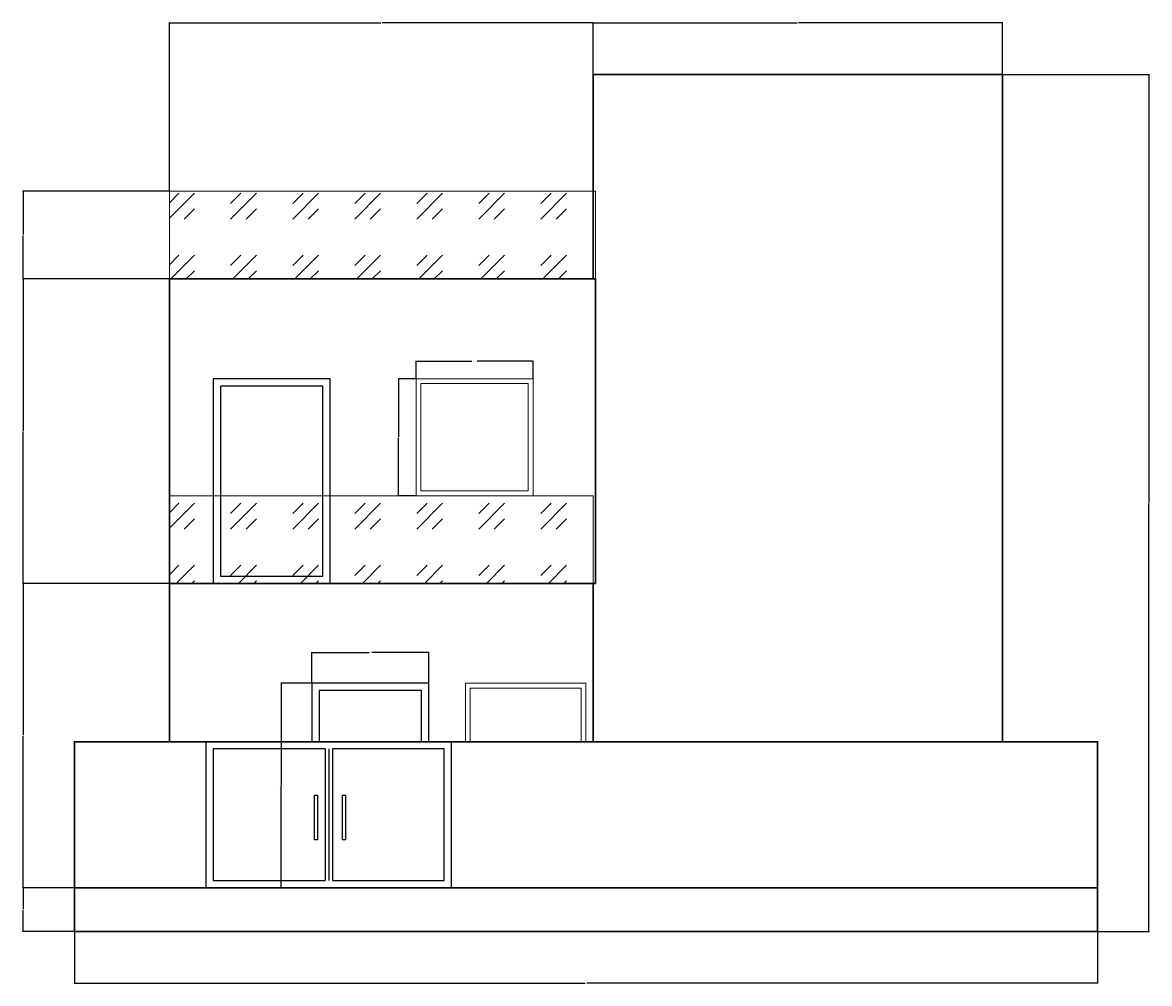
# Model space of a CAD drawing. Units: inches. Extents: x 810 to 2232, y 728 to 1827.
# Tile 4 of 6: x 1317 to 1780, y 1201 to 1596. Entities that reach past the tile are written whole.
import ezdxf

# ---------------------------------------------------------------- set-up
doc = ezdxf.new("R2010")
doc.units = ezdxf.units.IN
for name, color, linetype, lineweight in [('A-ANNO-DIMS', 2, 'Continuous', 18), ('A-ELEV', 7, 'Continuous', 30), ('A-ELEV-DOOR', 7, 'Continuous', 25), ('A-ELEV-GATE', 7, 'Continuous', 25), ('A-ELEV-GLAZ', 7, 'Continuous', 18), ('A-ELEV-PATT', 8, 'Continuous', 13), ('A-ELEV-SITE', 7, 'Continuous', 30)]:
    doc.layers.add(name, color=color, linetype=linetype, lineweight=lineweight)
doc.styles.get("Standard").update_dxf_attribs({"font": 'arial.ttf'})
doc.dimstyles.get("Standard").update_dxf_attribs({"dimtxt": 0.18, "dimasz": 0.18, "dimexe": 0.18, "dimexo": 0.0625, "dimgap": 0.09, "dimtad": 0, "dimtih": 1, "dimtoh": 1, "dimdec": 4, "dimzin": 0, "dimdsep": 46, "dimtxsty": 'Standard', "dimcen": 0.09, "dimadec": 0, "dimazin": 0, "dimtfac": 1, "dimtdec": 4, "dimtofl": 0, "dimtmove": 0, "dimatfit": 3, "dimfxl": 1, "dimtolj": 1, "dimtzin": 0, "dimarcsym": 0})
pattern_1 = [(45, (-481.11, 598.717), (25.45584, 0), [15, -21]), (45, (-474.746, 598.717), (25.45584, 0), [6, -30]), (45, (-481.11, 605.081), (25.45584, 0), [6, -30])]

# ---------------------------------------------------------------- blocks, each defined once
blk = doc.blocks.new('GATE-DOUBLE-ELEV')
for p, q in [((48.89, 57), (48.89, 3)), ((50.39, 57), (50.39, 3)), ((51.89, 57), (51.89, 3))]:
    blk.add_line(p, q)
for points in [[(0, 0), (100.77, 0), (100.77, 60), (0, 60)], [(44.48, 38.04), (45.81, 38.04), (45.81, 19.7), (44.48, 19.7)], [(55.99, 38.04), (57.32, 38.04), (57.32, 19.7), (55.99, 19.7)]]:
    blk.add_lwpolyline(points, close=True)
for points in [[(48.89, 57), (3, 57), (3, 3), (48.89, 3)], [(51.89, 3), (97.77, 3), (97.77, 57), (51.89, 57)]]:
    blk.add_lwpolyline(points)
blk = doc.blocks.new('DOOR-ENTRY-ELEV-SCREENED')
for points in [[(48, 60), (48, 84), (0, 84), (0, 60)], [(45, 60), (45, 81), (3, 81), (3, 60)], [(0, 0), (48, 0)]]:
    blk.add_lwpolyline(points)
blk = doc.blocks.new('WIN-ELEV-SCREENED')
for points in [[(0, 0), (0, 24), (49.5, 24), (49.5, 0)], [(2, 0), (2, 22), (47.5, 22), (47.5, 0)]]:
    blk.add_lwpolyline(points)
blk = doc.blocks.new('DOOR-BALCONY-ELEV')
for points in [[(0, 0), (48, 0), (48, 84), (0, 84)], [(3, 3), (45, 3), (45, 81), (3, 81)]]:
    blk.add_lwpolyline(points, close=True)
blk = doc.blocks.new('WIN-ELEV-SQUARE')
for points in [[(0, 0), (48, 0), (48, 48), (0, 48)], [(2, 2), (46, 2), (46, 46), (2, 46)]]:
    blk.add_lwpolyline(points, close=True)
blk = doc.blocks.new('*D43')
at = {"layer": 'A-ANNO-DIMS', "color": 0, "lineweight": -2, "transparency": 16777216}
for p, q in [((1435.94, 1324.56), (1423.23, 1324.56)), ((1423.41, 1324.38), (1423.41, 1282.74)), ((1423.41, 1240.74), (1423.41, 1282.37)), ((1435.94, 1240.56), (1423.23, 1240.56))]:
    blk.add_line(p, q, dxfattribs=at)
at = {"layer": 'A-ANNO-DIMS', "color": 0, "transparency": 16777216}
for points in [[(1423.38, 1324.38), (1423.44, 1324.38), (1423.41, 1324.56)], [(1423.38, 1240.74), (1423.44, 1240.74), (1423.41, 1240.56)]]:
    blk.add_solid(points, dxfattribs=at)
at = {"layer": 'Defpoints', "color": 0, "transparency": 16777216}
for p in [(1423.41, 1324.56), (1436.01, 1324.56), (1436.01, 1240.56)]:
    blk.add_point(p, dxfattribs=at)
at = {"layer": 'A-ANNO-DIMS', "color": 0, "transparency": 16777216, "insert": (1423.41, 1282.56), "char_height": 0.18, "attachment_point": 5}
blk.add_mtext('\\A1;ENTRY DOOR 84 TYP.', dxfattribs=at)
blk = doc.blocks.new('*D44')
at = {"layer": 'A-ANNO-DIMS', "color": 0, "lineweight": -2, "transparency": 16777216}
for p, q in [((1436.01, 1324.62), (1436.01, 1337.34)), ((1436.19, 1337.16), (1459.48, 1337.16)), ((1483.83, 1337.16), (1460.54, 1337.16)), ((1484.01, 1324.62), (1484.01, 1337.34))]:
    blk.add_line(p, q, dxfattribs=at)
at = {"layer": 'A-ANNO-DIMS', "color": 0, "transparency": 16777216}
for points in [[(1436.19, 1337.19), (1436.19, 1337.13), (1436.01, 1337.16)], [(1483.83, 1337.19), (1483.83, 1337.13), (1484.01, 1337.16)]]:
    blk.add_solid(points, dxfattribs=at)
at = {"layer": 'Defpoints', "color": 0, "transparency": 16777216}
for p in [(1484.01, 1337.16), (1436.01, 1324.56), (1484.01, 1324.56)]:
    blk.add_point(p, dxfattribs=at)
at = {"layer": 'A-ANNO-DIMS', "color": 0, "transparency": 16777216, "insert": (1460.01, 1337.16), "char_height": 0.18, "attachment_point": 5}
blk.add_mtext('\\A1;48 TYP.', dxfattribs=at)
blk = doc.blocks.new('*D49')
at = {"layer": 'A-ANNO-DIMS', "color": 0, "lineweight": -2, "transparency": 16777216}
for p, q in [((1478.76, 1449.62), (1478.76, 1456.94)), ((1478.94, 1456.76), (1501.64, 1456.76)), ((1526.58, 1456.76), (1503.88, 1456.76)), ((1526.76, 1449.62), (1526.76, 1456.94))]:
    blk.add_line(p, q, dxfattribs=at)
at = {"layer": 'A-ANNO-DIMS', "color": 0, "transparency": 16777216}
for points in [[(1478.94, 1456.79), (1478.94, 1456.73), (1478.76, 1456.76)], [(1526.58, 1456.79), (1526.58, 1456.73), (1526.76, 1456.76)]]:
    blk.add_solid(points, dxfattribs=at)
at = {"layer": 'Defpoints', "color": 0, "transparency": 16777216}
for p in [(1526.76, 1456.76), (1478.76, 1449.56), (1526.76, 1449.56)]:
    blk.add_point(p, dxfattribs=at)
at = {"layer": 'A-ANNO-DIMS', "color": 0, "transparency": 16777216, "insert": (1502.76, 1456.76), "char_height": 0.18, "attachment_point": 5}
blk.add_mtext('\\A1;WINDOW 48 TYP.', dxfattribs=at)
blk = doc.blocks.new('*D50')
at = {"layer": 'A-ANNO-DIMS', "color": 0, "lineweight": -2, "transparency": 16777216}
for p, q in [((1478.69, 1449.56), (1471.38, 1449.56)), ((1471.56, 1449.38), (1471.56, 1425.74)), ((1471.56, 1401.74), (1471.56, 1425.38)), ((1478.69, 1401.56), (1471.38, 1401.56))]:
    blk.add_line(p, q, dxfattribs=at)
at = {"layer": 'A-ANNO-DIMS', "color": 0, "transparency": 16777216}
for points in [[(1471.53, 1449.38), (1471.59, 1449.38), (1471.56, 1449.56)], [(1471.53, 1401.74), (1471.59, 1401.74), (1471.56, 1401.56)]]:
    blk.add_solid(points, dxfattribs=at)
at = {"layer": 'Defpoints', "color": 0, "transparency": 16777216}
for p in [(1471.56, 1449.56), (1478.76, 1449.56), (1478.76, 1401.56)]:
    blk.add_point(p, dxfattribs=at)
at = {"layer": 'A-ANNO-DIMS', "color": 0, "transparency": 16777216, "insert": (1471.56, 1425.56), "char_height": 0.18, "attachment_point": 5}
blk.add_mtext('\\A1;48 TYP.', dxfattribs=at)
blk = doc.blocks.new('*D75')
at = {"layer": 'A-ANNO-DIMS', "color": 0, "lineweight": -2, "transparency": 16777216}
for p, q in [((1338.51, 1222.5), (1338.51, 1201.28)), ((1758.51, 1222.5), (1758.51, 1201.28)), ((1338.69, 1201.46), (1548.21, 1201.46)), ((1758.33, 1201.46), (1548.8, 1201.46))]:
    blk.add_line(p, q, dxfattribs=at)
at = {"layer": 'A-ANNO-DIMS', "color": 0, "transparency": 16777216}
for points in [[(1338.69, 1201.49), (1338.69, 1201.43), (1338.51, 1201.46)], [(1758.33, 1201.49), (1758.33, 1201.43), (1758.51, 1201.46)]]:
    blk.add_solid(points, dxfattribs=at)
at = {"layer": 'Defpoints', "color": 0, "transparency": 16777216}
for p in [(1338.51, 1222.56), (1758.51, 1222.56), (1758.51, 1201.46)]:
    blk.add_point(p, dxfattribs=at)
at = {"layer": 'A-ANNO-DIMS', "color": 0, "transparency": 16777216, "insert": (1548.51, 1201.46), "char_height": 0.18, "attachment_point": 5}
blk.add_mtext('\\A1;420', dxfattribs=at)
blk = doc.blocks.new('*D76')
at = {"layer": 'A-ANNO-DIMS', "color": 0, "lineweight": -2, "transparency": 16777216}
for p, q in [((1719.57, 1574.56), (1779.79, 1574.56)), ((1779.61, 1574.38), (1779.61, 1398.74)), ((1779.61, 1222.74), (1779.61, 1398.38)), ((1758.57, 1222.56), (1779.79, 1222.56))]:
    blk.add_line(p, q, dxfattribs=at)
at = {"layer": 'A-ANNO-DIMS', "color": 0, "transparency": 16777216}
for points in [[(1779.58, 1574.38), (1779.64, 1574.38), (1779.61, 1574.56)], [(1779.58, 1222.74), (1779.64, 1222.74), (1779.61, 1222.56)]]:
    blk.add_solid(points, dxfattribs=at)
at = {"layer": 'Defpoints', "color": 0, "transparency": 16777216}
for p in [(1719.51, 1574.56), (1779.61, 1574.56), (1758.51, 1222.56)]:
    blk.add_point(p, dxfattribs=at)
at = {"layer": 'A-ANNO-DIMS', "color": 0, "transparency": 16777216, "insert": (1779.61, 1398.56), "char_height": 0.18, "attachment_point": 5}
blk.add_mtext('\\A1;352', dxfattribs=at)
blk = doc.blocks.new('*D77')
at = {"layer": 'A-ANNO-DIMS', "color": 0, "lineweight": -2, "transparency": 16777216}
for p, q in [((1338.44, 1240.56), (1317.23, 1240.56)), ((1317.41, 1240.38), (1317.41, 1231.74)), ((1317.41, 1222.74), (1317.41, 1231.38)), ((1338.44, 1222.56), (1317.23, 1222.56))]:
    blk.add_line(p, q, dxfattribs=at)
at = {"layer": 'A-ANNO-DIMS', "color": 0, "transparency": 16777216}
for points in [[(1317.38, 1240.38), (1317.44, 1240.38), (1317.41, 1240.56)], [(1317.38, 1222.74), (1317.44, 1222.74), (1317.41, 1222.56)]]:
    blk.add_solid(points, dxfattribs=at)
at = {"layer": 'Defpoints', "color": 0, "transparency": 16777216}
for p in [(1317.41, 1240.56), (1338.51, 1240.56), (1338.51, 1222.56)]:
    blk.add_point(p, dxfattribs=at)
at = {"layer": 'A-ANNO-DIMS', "color": 0, "transparency": 16777216, "insert": (1317.41, 1231.56), "char_height": 0.18, "attachment_point": 5}
blk.add_mtext('\\A1;18', dxfattribs=at)
blk = doc.blocks.new('*D78')
at = {"layer": 'A-ANNO-DIMS', "color": 0, "lineweight": -2, "transparency": 16777216}
for p, q in [((1377.44, 1365.56), (1317.23, 1365.56)), ((1317.41, 1365.38), (1317.41, 1303.24)), ((1317.41, 1240.74), (1317.41, 1302.88)), ((1338.44, 1240.56), (1317.23, 1240.56))]:
    blk.add_line(p, q, dxfattribs=at)
at = {"layer": 'A-ANNO-DIMS', "color": 0, "transparency": 16777216}
for points in [[(1317.38, 1365.38), (1317.44, 1365.38), (1317.41, 1365.56)], [(1317.38, 1240.74), (1317.44, 1240.74), (1317.41, 1240.56)]]:
    blk.add_solid(points, dxfattribs=at)
at = {"layer": 'Defpoints', "color": 0, "transparency": 16777216}
for p in [(1317.41, 1365.56), (1377.51, 1365.56), (1338.51, 1240.56)]:
    blk.add_point(p, dxfattribs=at)
at = {"layer": 'A-ANNO-DIMS', "color": 0, "transparency": 16777216, "insert": (1317.41, 1303.06), "char_height": 0.18, "attachment_point": 5}
blk.add_mtext('\\A1;125', dxfattribs=at)
blk = doc.blocks.new('*D79')
at = {"layer": 'A-ANNO-DIMS', "color": 0, "lineweight": -2, "transparency": 16777216}
for p, q in [((1377.44, 1490.56), (1317.23, 1490.56)), ((1317.41, 1490.38), (1317.41, 1428.24)), ((1317.41, 1365.74), (1317.41, 1427.88)), ((1377.44, 1365.56), (1317.23, 1365.56))]:
    blk.add_line(p, q, dxfattribs=at)
at = {"layer": 'A-ANNO-DIMS', "color": 0, "transparency": 16777216}
for points in [[(1317.38, 1490.38), (1317.44, 1490.38), (1317.41, 1490.56)], [(1317.38, 1365.74), (1317.44, 1365.74), (1317.41, 1365.56)]]:
    blk.add_solid(points, dxfattribs=at)
at = {"layer": 'Defpoints', "color": 0, "transparency": 16777216}
for p in [(1317.41, 1490.56), (1377.51, 1490.56), (1377.51, 1365.56)]:
    blk.add_point(p, dxfattribs=at)
at = {"layer": 'A-ANNO-DIMS', "color": 0, "transparency": 16777216, "insert": (1317.41, 1428.06), "char_height": 0.18, "attachment_point": 5}
blk.add_mtext('\\A1;125', dxfattribs=at)
blk = doc.blocks.new('*D80')
at = {"layer": 'A-ANNO-DIMS', "color": 0, "lineweight": -2, "transparency": 16777216}
for p, q in [((1377.44, 1526.56), (1317.23, 1526.56)), ((1317.41, 1526.38), (1317.41, 1508.74)), ((1317.41, 1490.74), (1317.41, 1508.38)), ((1377.44, 1490.56), (1317.23, 1490.56))]:
    blk.add_line(p, q, dxfattribs=at)
at = {"layer": 'A-ANNO-DIMS', "color": 0, "transparency": 16777216}
for points in [[(1317.38, 1526.38), (1317.44, 1526.38), (1317.41, 1526.56)], [(1317.38, 1490.74), (1317.44, 1490.74), (1317.41, 1490.56)]]:
    blk.add_solid(points, dxfattribs=at)
at = {"layer": 'Defpoints', "color": 0, "transparency": 16777216}
for p in [(1317.41, 1526.56), (1377.51, 1526.56), (1377.51, 1490.56)]:
    blk.add_point(p, dxfattribs=at)
at = {"layer": 'A-ANNO-DIMS', "color": 0, "transparency": 16777216, "insert": (1317.41, 1508.56), "char_height": 0.18, "attachment_point": 5}
blk.add_mtext('\\A1;36', dxfattribs=at)
blk = doc.blocks.new('*D81')
at = {"layer": 'A-ANNO-DIMS', "color": 0, "lineweight": -2, "transparency": 16777216}
for p, q in [((1377.51, 1526.62), (1377.51, 1595.84)), ((1377.69, 1595.66), (1464.23, 1595.66)), ((1551.33, 1595.66), (1464.79, 1595.66)), ((1551.51, 1574.62), (1551.51, 1595.84))]:
    blk.add_line(p, q, dxfattribs=at)
at = {"layer": 'A-ANNO-DIMS', "color": 0, "transparency": 16777216}
for points in [[(1377.69, 1595.69), (1377.69, 1595.63), (1377.51, 1595.66)], [(1551.33, 1595.69), (1551.33, 1595.63), (1551.51, 1595.66)]]:
    blk.add_solid(points, dxfattribs=at)
at = {"layer": 'Defpoints', "color": 0, "transparency": 16777216}
for p in [(1551.51, 1595.66), (1551.51, 1574.56), (1377.51, 1526.56)]:
    blk.add_point(p, dxfattribs=at)
at = {"layer": 'A-ANNO-DIMS', "color": 0, "transparency": 16777216, "insert": (1464.51, 1595.66), "char_height": 0.18, "attachment_point": 5}
blk.add_mtext('\\A1;174', dxfattribs=at)
blk = doc.blocks.new('*D82')
at = {"layer": 'A-ANNO-DIMS', "color": 0, "lineweight": -2, "transparency": 16777216}
for p, q in [((1551.51, 1574.62), (1551.51, 1595.84)), ((1551.69, 1595.66), (1635.23, 1595.66)), ((1719.33, 1595.66), (1635.79, 1595.66)), ((1719.51, 1574.62), (1719.51, 1595.84))]:
    blk.add_line(p, q, dxfattribs=at)
at = {"layer": 'A-ANNO-DIMS', "color": 0, "transparency": 16777216}
for points in [[(1551.69, 1595.69), (1551.69, 1595.63), (1551.51, 1595.66)], [(1719.33, 1595.69), (1719.33, 1595.63), (1719.51, 1595.66)]]:
    blk.add_solid(points, dxfattribs=at)
at = {"layer": 'Defpoints', "color": 0, "transparency": 16777216}
for p in [(1719.51, 1595.66), (1551.51, 1574.56), (1719.51, 1574.56)]:
    blk.add_point(p, dxfattribs=at)
at = {"layer": 'A-ANNO-DIMS', "color": 0, "transparency": 16777216, "insert": (1635.51, 1595.66), "char_height": 0.18, "attachment_point": 5}
blk.add_mtext('\\A1;168', dxfattribs=at)

msp = doc.modelspace()

# ---------------------------------------------------------------- hatches: boundary and pattern name
at = {"layer": 'A-ELEV-PATT'}
h = msp.add_hatch(dxfattribs=at)
h.set_pattern_fill('GOST_GLASS', color=256, scale=3)
h.set_pattern_definition(pattern_1)
h.paths.add_polyline_path([(1552.3502, 1490.5577), (1377.5068, 1490.5577), (1377.5068, 1526.5577), (1552.3502, 1526.5577)])
h = msp.add_hatch(dxfattribs=at)
h.set_pattern_fill('GOST_GLASS', color=256, scale=3)
h.set_pattern_definition(pattern_1)
h.paths.add_polyline_path([(1377.5068, 1365.5577), (1551.5068, 1365.5577), (1551.5068, 1401.5577), (1377.5068, 1401.5577)])

# ---------------------------------------------------------------- linework, layer by layer
at = {"layer": 'A-ELEV'}
for points in [[(1552.3502, 1490.5577), (1551.5068, 1490.5577), (1551.5068, 1574.5577), (1719.5068, 1574.5577), (1719.5068, 1490.5577)], [(1719.5068, 1526.5577), (1719.5068, 1490.5577)], [(1552.3502, 1365.5577), (1552.3502, 1490.5577)], [(1719.5068, 1490.5577), (1719.5068, 1365.5577)], [(1551.5068, 1300.5577), (1551.5068, 1365.5577), (1377.5068, 1365.5577), (1377.5068, 1300.5577)], [(1551.5068, 1300.5577), (1551.5068, 1365.5577), (1552.3502, 1365.5577)], [(1719.5068, 1365.5577), (1719.5068, 1300.5577)], [(1377.5068, 1240.5577), (1551.5068, 1240.5577)], [(1719.5068, 1240.5577), (1551.5068, 1240.5577)]]:
    msp.add_lwpolyline(points, dxfattribs=at)
msp.add_lwpolyline([(1377.5068, 1365.5577), (1552.3502, 1365.5577), (1552.3502, 1490.5577), (1377.5068, 1490.5577)], close=True, dxfattribs=at)
at = {"layer": 'A-ELEV-GLAZ'}
for points in [[(1552.3502, 1490.5577), (1377.5068, 1490.5577), (1377.5068, 1526.5577), (1552.3502, 1526.5577)], [(1377.5068, 1365.5577), (1551.5068, 1365.5577), (1551.5068, 1401.5577), (1377.5068, 1401.5577)]]:
    msp.add_lwpolyline(points, close=True, dxfattribs=at)
at = {"layer": 'A-ELEV-SITE'}
for points in [[(1338.5068, 1240.5577), (1758.5068, 1240.5577), (1758.5068, 1300.5577), (1338.5068, 1300.5577)], [(1338.5068, 1240.5577), (1758.5068, 1240.5577), (1758.5068, 1222.5577), (1338.5068, 1222.5577)]]:
    msp.add_lwpolyline(points, close=True, dxfattribs=at)

# ---------------------------------------------------------------- block references
at = {"layer": 'A-ELEV-DOOR'}
for name, p in [('DOOR-BALCONY-ELEV', (1395.5068, 1365.5581)), ('DOOR-ENTRY-ELEV-SCREENED', (1436.0067, 1240.5581))]:
    msp.add_blockref(name, p, dxfattribs=at)
at = {"layer": 'A-ELEV-GATE'}
msp.add_blockref('GATE-DOUBLE-ELEV', (1392.5067, 1240.5581), dxfattribs=at)
at = {"layer": 'A-ELEV-GLAZ'}
for name, p in [('WIN-ELEV-SQUARE', (1478.7568, 1401.5581)), ('WIN-ELEV-SCREENED', (1499.0067, 1300.5581))]:
    msp.add_blockref(name, p, dxfattribs=at)

# ---------------------------------------------------------------- dimensions: what is measured, and where the dimension line sits
at = {"layer": 'A-ANNO-DIMS'}
for base, p1, p2, picture, middle in [((1551.5068, 1595.6577), (1377.5068, 1526.5577), (1551.5068, 1574.5577), '*D81', (1464.5068, 1595.6577)), ((1719.5068, 1595.6577), (1551.5068, 1574.5577), (1719.5068, 1574.5577), '*D82', (1635.5068, 1595.6577)), ((1758.5068, 1201.4577), (1338.5068, 1222.5577), (1758.5068, 1222.5577), '*D75', (1548.5068, 1201.4577))]:
    dim = msp.add_linear_dim(base=base, p1=p1, p2=p2, dimstyle='Standard', override={"dimdec": 0, "dimlfac": 1, "dimrnd": 0, "dimzin": 0, "dimdsep": 46, "dimlunit": 2}, dxfattribs=at)
    dim.commit()
    dim.dimension.update_dxf_attribs({"geometry": picture, "text_midpoint": middle})
for base, p1, p2, picture, middle in [((1779.6068, 1574.5577), (1758.5068, 1222.5577), (1719.5068, 1574.5577), '*D76', (1779.6068, 1398.5577)), ((1317.4068, 1526.5577), (1377.5068, 1490.5577), (1377.5068, 1526.5577), '*D80', (1317.4068, 1508.5577)), ((1317.4068, 1490.5577), (1377.5068, 1365.5577), (1377.5068, 1490.5577), '*D79', (1317.4068, 1428.0577)), ((1317.4068, 1365.5577), (1338.5068, 1240.5577), (1377.5068, 1365.5577), '*D78', (1317.4068, 1303.0577)), ((1317.4068, 1240.5577), (1338.5068, 1222.5577), (1338.5068, 1240.5577), '*D77', (1317.4068, 1231.5577))]:
    dim = msp.add_linear_dim(base=base, p1=p1, p2=p2, angle=90, dimstyle='Standard', override={"dimdec": 0, "dimlfac": 1, "dimrnd": 0, "dimzin": 0, "dimdsep": 46, "dimlunit": 2}, dxfattribs=at)
    dim.commit()
    dim.dimension.update_dxf_attribs({"geometry": picture, "text_midpoint": middle})
for base, p1, p2, text, picture, middle in [((1526.7568, 1456.7577), (1478.7568, 1449.5577), (1526.7568, 1449.5577), 'WINDOW <> TYP.', '*D49', (1502.7568, 1456.7577)), ((1484.0068, 1337.1577), (1436.0068, 1324.5577), (1484.0068, 1324.5577), '<> TYP.', '*D44', (1460.0068, 1337.1577))]:
    dim = msp.add_linear_dim(base=base, p1=p1, p2=p2, text=text, dimstyle='Standard', override={"dimdec": 0, "dimlfac": 1, "dimrnd": 0, "dimzin": 0, "dimdsep": 46, "dimlunit": 2}, dxfattribs=at)
    dim.commit()
    dim.dimension.update_dxf_attribs({"geometry": picture, "text_midpoint": middle})
for base, p1, p2, text, picture, middle in [((1471.5568, 1449.5577), (1478.7568, 1401.5577), (1478.7568, 1449.5577), '<> TYP.', '*D50', (1471.5568, 1425.5577)), ((1423.4068, 1324.5577), (1436.0068, 1240.5577), (1436.0068, 1324.5577), 'ENTRY DOOR <> TYP.', '*D43', (1423.4068, 1282.5577))]:
    dim = msp.add_linear_dim(base=base, p1=p1, p2=p2, angle=90, text=text, dimstyle='Standard', override={"dimdec": 0, "dimlfac": 1, "dimrnd": 0, "dimzin": 0, "dimdsep": 46, "dimlunit": 2}, dxfattribs=at)
    dim.commit()
    dim.dimension.update_dxf_attribs({"geometry": picture, "text_midpoint": middle})

doc.saveas('drawing.dxf')
